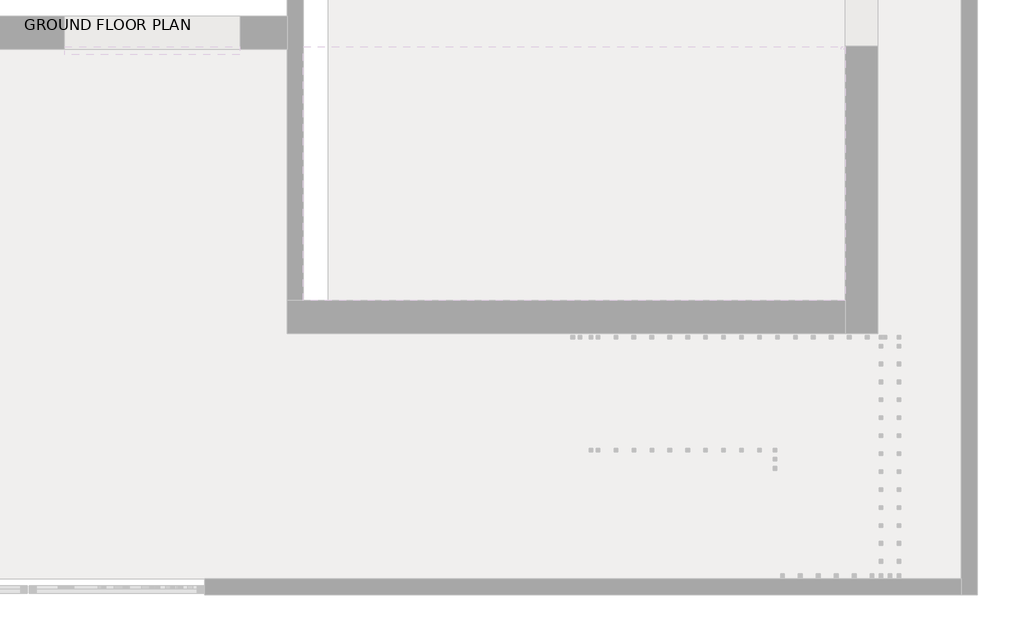
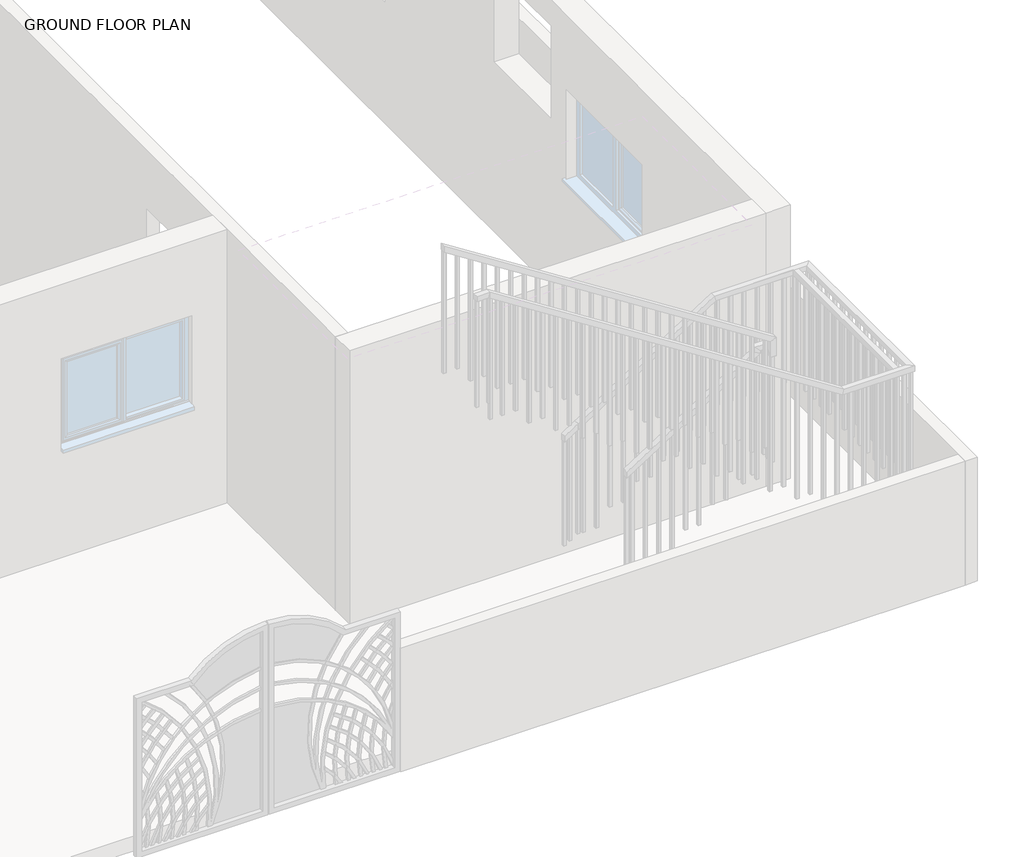
# One storey, part 16 of 23: 2 railings.
"""IFC4 building model written with IfcOpenShell, lengths in millimetres."""

from ifc_helpers import new_model, si_unit, frame, origin, place, context, project, spatial, polyline, outline, extrude, faceted_brep, element, save

model = new_model("IFC4")

# Units and contexts
model_context = context("Model", 3, world=origin())
ifc_project = project(units=[si_unit("LENGTHUNIT", "METRE", prefix="MILLI")], contexts=[model_context])

# Site, building, storey
site = spatial("IfcSite", under=ifc_project)
building = spatial("IfcBuilding", under=site)
storey = spatial("IfcBuildingStorey", under=building, Name="GROUND FLOOR PLAN", Elevation=487.68)

# Railings
placement = place(None, origin())
element("IfcRailing", 1, ObjectType="1100mm", at=placement, inside=storey, context=model_context, shape_type="SolidModel", body=[
    faceted_brep([(-8680.149573, -10220.0521308, 1912.8), (-8680.149573, -10220.0521308, 1853.4423995), (-8680.149573, -10270.0521308, 1853.4423995), (-8680.149573, -10270.0521308, 1912.8), (-7409.7306254, -10220.0521308, 2725.6), (-7395.1045513, -10220.0521308, 2675.6), (-7395.1045513, -10270.0521308, 2675.6), (-7409.7306254, -10270.0521308, 2725.6), (-6495.8132565, -10220.0521308, 2725.6), (-6495.8132565, -10220.0521308, 2675.6), (-6545.8132565, -10270.0521308, 2675.6), (-6545.8132565, -10270.0521308, 2725.6), (-6495.8132565, -11933.6860066, 2725.6), (-6495.8132565, -11933.6860066, 2675.6), (-6545.8132565, -11883.6860066, 2675.6), (-6545.8132565, -11883.6860066, 2725.6), (-7155.718398, -11933.6860066, 2725.6), (-7170.3479429, -11933.6860066, 2675.6), (-7170.3479429, -11883.6860066, 2675.6), (-7155.718398, -11883.6860066, 2725.6), (-10457.8773536, -11933.6860066, 4838.88), (-10457.8773536, -11883.6860066, 4838.88), (-10457.8773536, -11883.6860066, 4779.517542), (-10457.8773536, -11933.6860066, 4779.517542)], [[[0, 1, 2, 3]], [[1, 0, 4, 5]], [[2, 1, 5, 6]], [[3, 2, 6, 7]], [[0, 3, 7, 4]], [[5, 4, 8, 9]], [[6, 5, 9, 10]], [[7, 6, 10, 11]], [[4, 7, 11, 8]], [[9, 8, 12, 13]], [[10, 9, 13, 14]], [[11, 10, 14, 15]], [[8, 11, 15, 12]], [[13, 12, 16, 17]], [[14, 13, 17, 18]], [[15, 14, 18, 19]], [[12, 15, 19, 16]], [[20, 21, 22, 23]], [[17, 16, 20, 23]], [[18, 17, 23, 22]], [[19, 18, 22, 21]], [[16, 19, 21, 20]]]),
    extrude(outline(polyline([(4691.8007425, -10320.8132565), (4707.7999723, -10345.8132565), (3576.32, -10345.8132565), (3576.32, -10320.8132565), (4691.8007425, -10320.8132565)])), frame((0.0, -11921.1860066, 0.0), z_axis=(0.0, 1.0, 0.0), x_axis=(0.0, 0.0, 1.0)), (0.0, 0.0, 1.0), 25.0),
    extrude(outline(polyline([(4611.8045935, -10195.8132565), (4627.8038233, -10220.8132565), (3576.32, -10220.8132565), (3576.32, -10195.8132565), (4611.8045935, -10195.8132565)])), frame((0.0, -11921.1860066, 0.0), z_axis=(0.0, 1.0, 0.0), x_axis=(0.0, 0.0, 1.0)), (0.0, 0.0, 1.0), 25.0),
    extrude(outline(polyline([(4531.8084444, -10070.8132565), (4547.8076742, -10095.8132565), (3413.76, -10095.8132565), (3413.76, -10070.8132565), (4531.8084444, -10070.8132565)])), frame((0.0, -11921.1860066, 0.0), z_axis=(0.0, 1.0, 0.0), x_axis=(0.0, 0.0, 1.0)), (0.0, 0.0, 1.0), 25.0),
    extrude(outline(polyline([(4451.8122954, -9945.8132565), (4467.8115252, -9970.8132565), (3413.76, -9970.8132565), (3413.76, -9945.8132565), (4451.8122954, -9945.8132565)])), frame((0.0, -11921.1860066, 0.0), z_axis=(0.0, 1.0, 0.0), x_axis=(0.0, 0.0, 1.0)), (0.0, 0.0, 1.0), 25.0),
    extrude(outline(polyline([(4371.8161463, -9820.8132565), (4387.8153761, -9845.8132565), (3251.2, -9845.8132565), (3251.2, -9820.8132565), (4371.8161463, -9820.8132565)])), frame((0.0, -11921.1860066, 0.0), z_axis=(0.0, 1.0, 0.0), x_axis=(0.0, 0.0, 1.0)), (0.0, 0.0, 1.0), 25.0),
    extrude(outline(polyline([(4291.8423995, -9695.8132565), (4307.8371231, -9720.8132565), (3251.2, -9720.8132565), (3251.2, -9695.8132565), (4291.8423995, -9695.8132565)])), frame((0.0, -11921.1860066, 0.0), z_axis=(0.0, 1.0, 0.0), x_axis=(0.0, 0.0, 1.0)), (0.0, 0.0, 1.0), 25.0),
    extrude(outline(polyline([(4211.8238482, -9570.8132565), (4227.823078, -9595.8132565), (3088.64, -9595.8132565), (3088.64, -9570.8132565), (4211.8238482, -9570.8132565)])), frame((0.0, -11921.1860066, 0.0), z_axis=(0.0, 1.0, 0.0), x_axis=(0.0, 0.0, 1.0)), (0.0, 0.0, 1.0), 25.0),
    extrude(outline(polyline([(4131.8276992, -9445.8132565), (4147.826929, -9470.8132565), (3088.64, -9470.8132565), (3088.64, -9445.8132565), (4131.8276992, -9445.8132565)])), frame((0.0, -11921.1860066, 0.0), z_axis=(0.0, 1.0, 0.0), x_axis=(0.0, 0.0, 1.0)), (0.0, 0.0, 1.0), 25.0),
    extrude(outline(polyline([(4051.8315501, -9320.8132565), (4067.8307799, -9345.8132565), (2926.08, -9345.8132565), (2926.08, -9320.8132565), (4051.8315501, -9320.8132565)])), frame((0.0, -11921.1860066, 0.0), z_axis=(0.0, 1.0, 0.0), x_axis=(0.0, 0.0, 1.0)), (0.0, 0.0, 1.0), 25.0),
    extrude(outline(polyline([(3971.835401, -9195.8132565), (3987.8346309, -9220.8132565), (2926.08, -9220.8132565), (2926.08, -9195.8132565), (3971.835401, -9195.8132565)])), frame((0.0, -11921.1860066, 0.0), z_axis=(0.0, 1.0, 0.0), x_axis=(0.0, 0.0, 1.0)), (0.0, 0.0, 1.0), 25.0),
    extrude(outline(polyline([(3891.839252, -9070.8132565), (3907.8384818, -9095.8132565), (2763.52, -9095.8132565), (2763.52, -9070.8132565), (3891.839252, -9070.8132565)])), frame((0.0, -11921.1860066, 0.0), z_axis=(0.0, 1.0, 0.0), x_axis=(0.0, 0.0, 1.0)), (0.0, 0.0, 1.0), 25.0),
    extrude(outline(polyline([(3811.8431029, -8945.8132565), (3827.8423328, -8970.8132565), (2763.52, -8970.8132565), (2763.52, -8945.8132565), (3811.8431029, -8945.8132565)])), frame((0.0, -11921.1860066, 0.0), z_axis=(0.0, 1.0, 0.0), x_axis=(0.0, 0.0, 1.0)), (0.0, 0.0, 1.0), 25.0),
    extrude(outline(polyline([(3731.8469539, -8820.8132565), (3747.8461837, -8845.8132565), (2600.96, -8845.8132565), (2600.96, -8820.8132565), (3731.8469539, -8820.8132565)])), frame((0.0, -11921.1860066, 0.0), z_axis=(0.0, 1.0, 0.0), x_axis=(0.0, 0.0, 1.0)), (0.0, 0.0, 1.0), 25.0),
    extrude(outline(polyline([(3651.8508048, -8695.8132565), (3667.8500347, -8720.8132565), (2600.96, -8720.8132565), (2600.96, -8695.8132565), (3651.8508048, -8695.8132565)])), frame((0.0, -11921.1860066, 0.0), z_axis=(0.0, 1.0, 0.0), x_axis=(0.0, 0.0, 1.0)), (0.0, 0.0, 1.0), 25.0),
    extrude(outline(polyline([(3571.8546558, -8570.8132565), (3587.8538856, -8595.8132565), (2438.4, -8595.8132565), (2438.4, -8570.8132565), (3571.8546558, -8570.8132565)])), frame((0.0, -11921.1860066, 0.0), z_axis=(0.0, 1.0, 0.0), x_axis=(0.0, 0.0, 1.0)), (0.0, 0.0, 1.0), 25.0),
    extrude(outline(polyline([(3491.8585067, -8445.8132565), (3507.8577365, -8470.8132565), (2438.4, -8470.8132565), (2438.4, -8445.8132565), (3491.8585067, -8445.8132565)])), frame((0.0, -11921.1860066, 0.0), z_axis=(0.0, 1.0, 0.0), x_axis=(0.0, 0.0, 1.0)), (0.0, 0.0, 1.0), 25.0),
    extrude(outline(polyline([(3411.8623577, -8320.8132565), (3427.8615875, -8345.8132565), (2275.84, -8345.8132565), (2275.84, -8320.8132565), (3411.8623577, -8320.8132565)])), frame((0.0, -11921.1860066, 0.0), z_axis=(0.0, 1.0, 0.0), x_axis=(0.0, 0.0, 1.0)), (0.0, 0.0, 1.0), 25.0),
    extrude(outline(polyline([(3331.8662086, -8195.8132565), (3347.8654384, -8220.8132565), (2275.84, -8220.8132565), (2275.84, -8195.8132565), (3331.8662086, -8195.8132565)])), frame((0.0, -11921.1860066, 0.0), z_axis=(0.0, 1.0, 0.0), x_axis=(0.0, 0.0, 1.0)), (0.0, 0.0, 1.0), 25.0),
    extrude(outline(polyline([(3251.8700596, -8070.8132565), (3267.8692894, -8095.8132565), (2113.28, -8095.8132565), (2113.28, -8070.8132565), (3251.8700596, -8070.8132565)])), frame((0.0, -11921.1860066, 0.0), z_axis=(0.0, 1.0, 0.0), x_axis=(0.0, 0.0, 1.0)), (0.0, 0.0, 1.0), 25.0),
    extrude(outline(polyline([(3171.8739105, -7945.8132565), (3187.8731403, -7970.8132565), (2113.28, -7970.8132565), (2113.28, -7945.8132565), (3171.8739105, -7945.8132565)])), frame((0.0, -11921.1860066, 0.0), z_axis=(0.0, 1.0, 0.0), x_axis=(0.0, 0.0, 1.0)), (0.0, 0.0, 1.0), 25.0),
    extrude(outline(polyline([(3091.8777615, -7820.8132565), (3107.8769913, -7845.8132565), (1950.72, -7845.8132565), (1950.72, -7820.8132565), (3091.8777615, -7820.8132565)])), frame((0.0, -11921.1860066, 0.0), z_axis=(0.0, 1.0, 0.0), x_axis=(0.0, 0.0, 1.0)), (0.0, 0.0, 1.0), 25.0),
    extrude(outline(polyline([(3011.8816124, -7695.8132565), (3027.8808422, -7720.8132565), (1950.72, -7720.8132565), (1950.72, -7695.8132565), (3011.8816124, -7695.8132565)])), frame((0.0, -11921.1860066, 0.0), z_axis=(0.0, 1.0, 0.0), x_axis=(0.0, 0.0, 1.0)), (0.0, 0.0, 1.0), 25.0),
    extrude(outline(polyline([(2931.8854634, -7570.8132565), (2947.8846932, -7595.8132565), (1788.16, -7595.8132565), (1788.16, -7570.8132565), (2931.8854634, -7570.8132565)])), frame((0.0, -11921.1860066, 0.0), z_axis=(0.0, 1.0, 0.0), x_axis=(0.0, 0.0, 1.0)), (0.0, 0.0, 1.0), 25.0),
    extrude(outline(polyline([(2851.8893143, -7445.8132565), (2867.8885441, -7470.8132565), (1788.16, -7470.8132565), (1788.16, -7445.8132565), (2851.8893143, -7445.8132565)])), frame((0.0, -11921.1860066, 0.0), z_axis=(0.0, 1.0, 0.0), x_axis=(0.0, 0.0, 1.0)), (0.0, 0.0, 1.0), 25.0),
    extrude(outline(polyline([(2771.8931653, -7320.8132565), (2787.8923951, -7345.8132565), (1625.6, -7345.8132565), (1625.6, -7320.8132565), (2771.8931653, -7320.8132565)])), frame((0.0, -11921.1860066, 0.0), z_axis=(0.0, 1.0, 0.0), x_axis=(0.0, 0.0, 1.0)), (0.0, 0.0, 1.0), 25.0),
    extrude(outline(polyline([(2691.8970162, -7195.8132565), (2707.896246, -7220.8132565), (1625.6, -7220.8132565), (1625.6, -7195.8132565), (2691.8970162, -7195.8132565)])), frame((0.0, -11921.1860066, 0.0), z_axis=(0.0, 1.0, 0.0), x_axis=(0.0, 0.0, 1.0)), (0.0, 0.0, 1.0), 25.0),
    extrude(outline(polyline([(-7070.8132565, -11921.1860066), (-7095.8132565, -11921.1860066), (-7095.8132565, -11896.1860066), (-7070.8132565, -11896.1860066), (-7070.8132565, -11921.1860066)])), frame((0.0, 0.0, 1625.6), z_axis=(0.0, 0.0, 1.0), x_axis=(1.0, 0.0, 0.0)), (0.0, 0.0, 1.0), 1050.0),
    extrude(outline(polyline([(-6945.8132565, -11921.1860066), (-6970.8132565, -11921.1860066), (-6970.8132565, -11896.1860066), (-6945.8132565, -11896.1860066), (-6945.8132565, -11921.1860066)])), frame((0.0, 0.0, 1625.6), z_axis=(0.0, 0.0, 1.0), x_axis=(1.0, 0.0, 0.0)), (0.0, 0.0, 1.0), 1050.0),
    extrude(outline(polyline([(-6820.8132565, -11921.1860066), (-6845.8132565, -11921.1860066), (-6845.8132565, -11896.1860066), (-6820.8132565, -11896.1860066), (-6820.8132565, -11921.1860066)])), frame((0.0, 0.0, 1625.6), z_axis=(0.0, 0.0, 1.0), x_axis=(1.0, 0.0, 0.0)), (0.0, 0.0, 1.0), 1050.0),
    extrude(outline(polyline([(-6695.8132565, -11921.1860066), (-6720.8132565, -11921.1860066), (-6720.8132565, -11896.1860066), (-6695.8132565, -11896.1860066), (-6695.8132565, -11921.1860066)])), frame((0.0, 0.0, 1625.6), z_axis=(0.0, 0.0, 1.0), x_axis=(1.0, 0.0, 0.0)), (0.0, 0.0, 1.0), 1050.0),
    extrude(outline(polyline([(-6570.8132565, -11921.1860066), (-6595.8132565, -11921.1860066), (-6595.8132565, -11896.1860066), (-6570.8132565, -11896.1860066), (-6570.8132565, -11921.1860066)])), frame((0.0, 0.0, 1625.6), z_axis=(0.0, 0.0, 1.0), x_axis=(1.0, 0.0, 0.0)), (0.0, 0.0, 1.0), 1050.0),
    extrude(outline(polyline([(-6508.3132565, -11795.0521308), (-6508.3132565, -11820.0521308), (-6533.3132565, -11820.0521308), (-6533.3132565, -11795.0521308), (-6508.3132565, -11795.0521308)])), frame((0.0, 0.0, 1625.6), z_axis=(0.0, 0.0, 1.0), x_axis=(1.0, 0.0, 0.0)), (0.0, 0.0, 1.0), 1050.0),
    extrude(outline(polyline([(-6508.3132565, -11670.0521308), (-6508.3132565, -11695.0521308), (-6533.3132565, -11695.0521308), (-6533.3132565, -11670.0521308), (-6508.3132565, -11670.0521308)])), frame((0.0, 0.0, 1625.6), z_axis=(0.0, 0.0, 1.0), x_axis=(1.0, 0.0, 0.0)), (0.0, 0.0, 1.0), 1050.0),
    extrude(outline(polyline([(-6508.3132565, -11545.0521308), (-6508.3132565, -11570.0521308), (-6533.3132565, -11570.0521308), (-6533.3132565, -11545.0521308), (-6508.3132565, -11545.0521308)])), frame((0.0, 0.0, 1625.6), z_axis=(0.0, 0.0, 1.0), x_axis=(1.0, 0.0, 0.0)), (0.0, 0.0, 1.0), 1050.0),
    extrude(outline(polyline([(-6508.3132565, -11420.0521308), (-6508.3132565, -11445.0521308), (-6533.3132565, -11445.0521308), (-6533.3132565, -11420.0521308), (-6508.3132565, -11420.0521308)])), frame((0.0, 0.0, 1625.6), z_axis=(0.0, 0.0, 1.0), x_axis=(1.0, 0.0, 0.0)), (0.0, 0.0, 1.0), 1050.0),
    extrude(outline(polyline([(-6508.3132565, -11295.0521308), (-6508.3132565, -11320.0521308), (-6533.3132565, -11320.0521308), (-6533.3132565, -11295.0521308), (-6508.3132565, -11295.0521308)])), frame((0.0, 0.0, 1625.6), z_axis=(0.0, 0.0, 1.0), x_axis=(1.0, 0.0, 0.0)), (0.0, 0.0, 1.0), 1050.0),
    extrude(outline(polyline([(-6508.3132565, -11170.0521308), (-6508.3132565, -11195.0521308), (-6533.3132565, -11195.0521308), (-6533.3132565, -11170.0521308), (-6508.3132565, -11170.0521308)])), frame((0.0, 0.0, 1625.6), z_axis=(0.0, 0.0, 1.0), x_axis=(1.0, 0.0, 0.0)), (0.0, 0.0, 1.0), 1050.0),
    extrude(outline(polyline([(-6508.3132565, -11045.0521308), (-6508.3132565, -11070.0521308), (-6533.3132565, -11070.0521308), (-6533.3132565, -11045.0521308), (-6508.3132565, -11045.0521308)])), frame((0.0, 0.0, 1625.6), z_axis=(0.0, 0.0, 1.0), x_axis=(1.0, 0.0, 0.0)), (0.0, 0.0, 1.0), 1050.0),
    extrude(outline(polyline([(-6508.3132565, -10920.0521308), (-6508.3132565, -10945.0521308), (-6533.3132565, -10945.0521308), (-6533.3132565, -10920.0521308), (-6508.3132565, -10920.0521308)])), frame((0.0, 0.0, 1625.6), z_axis=(0.0, 0.0, 1.0), x_axis=(1.0, 0.0, 0.0)), (0.0, 0.0, 1.0), 1050.0),
    extrude(outline(polyline([(-6508.3132565, -10795.0521308), (-6508.3132565, -10820.0521308), (-6533.3132565, -10820.0521308), (-6533.3132565, -10795.0521308), (-6508.3132565, -10795.0521308)])), frame((0.0, 0.0, 1625.6), z_axis=(0.0, 0.0, 1.0), x_axis=(1.0, 0.0, 0.0)), (0.0, 0.0, 1.0), 1050.0),
    extrude(outline(polyline([(-6508.3132565, -10670.0521308), (-6508.3132565, -10695.0521308), (-6533.3132565, -10695.0521308), (-6533.3132565, -10670.0521308), (-6508.3132565, -10670.0521308)])), frame((0.0, 0.0, 1625.6), z_axis=(0.0, 0.0, 1.0), x_axis=(1.0, 0.0, 0.0)), (0.0, 0.0, 1.0), 1050.0),
    extrude(outline(polyline([(-6508.3132565, -10545.0521308), (-6508.3132565, -10570.0521308), (-6533.3132565, -10570.0521308), (-6533.3132565, -10545.0521308), (-6508.3132565, -10545.0521308)])), frame((0.0, 0.0, 1625.6), z_axis=(0.0, 0.0, 1.0), x_axis=(1.0, 0.0, 0.0)), (0.0, 0.0, 1.0), 1050.0),
    extrude(outline(polyline([(-6508.3132565, -10420.0521308), (-6508.3132565, -10445.0521308), (-6533.3132565, -10445.0521308), (-6533.3132565, -10420.0521308), (-6508.3132565, -10420.0521308)])), frame((0.0, 0.0, 1625.6), z_axis=(0.0, 0.0, 1.0), x_axis=(1.0, 0.0, 0.0)), (0.0, 0.0, 1.0), 1050.0),
    extrude(outline(polyline([(-6508.3132565, -10295.0521308), (-6508.3132565, -10320.0521308), (-6533.3132565, -10320.0521308), (-6533.3132565, -10295.0521308), (-6508.3132565, -10295.0521308)])), frame((0.0, 0.0, 1625.6), z_axis=(0.0, 0.0, 1.0), x_axis=(1.0, 0.0, 0.0)), (0.0, 0.0, 1.0), 1050.0),
    extrude(outline(polyline([(-6630.149573, -10232.5521308), (-6605.149573, -10232.5521308), (-6605.149573, -10257.5521308), (-6630.149573, -10257.5521308), (-6630.149573, -10232.5521308)])), frame((0.0, 0.0, 1625.6), z_axis=(0.0, 0.0, 1.0), x_axis=(1.0, 0.0, 0.0)), (0.0, 0.0, 1.0), 1050.0),
    extrude(outline(polyline([(-6755.149573, -10232.5521308), (-6730.149573, -10232.5521308), (-6730.149573, -10257.5521308), (-6755.149573, -10257.5521308), (-6755.149573, -10232.5521308)])), frame((0.0, 0.0, 1625.6), z_axis=(0.0, 0.0, 1.0), x_axis=(1.0, 0.0, 0.0)), (0.0, 0.0, 1.0), 1050.0),
    extrude(outline(polyline([(-6880.149573, -10232.5521308), (-6855.149573, -10232.5521308), (-6855.149573, -10257.5521308), (-6880.149573, -10257.5521308), (-6880.149573, -10232.5521308)])), frame((0.0, 0.0, 1625.6), z_axis=(0.0, 0.0, 1.0), x_axis=(1.0, 0.0, 0.0)), (0.0, 0.0, 1.0), 1050.0),
    extrude(outline(polyline([(-7005.149573, -10232.5521308), (-6980.149573, -10232.5521308), (-6980.149573, -10257.5521308), (-7005.149573, -10257.5521308), (-7005.149573, -10232.5521308)])), frame((0.0, 0.0, 1625.6), z_axis=(0.0, 0.0, 1.0), x_axis=(1.0, 0.0, 0.0)), (0.0, 0.0, 1.0), 1050.0),
    extrude(outline(polyline([(-7130.149573, -10232.5521308), (-7105.149573, -10232.5521308), (-7105.149573, -10257.5521308), (-7130.149573, -10257.5521308), (-7130.149573, -10232.5521308)])), frame((0.0, 0.0, 1625.6), z_axis=(0.0, 0.0, 1.0), x_axis=(1.0, 0.0, 0.0)), (0.0, 0.0, 1.0), 1050.0),
    extrude(outline(polyline([(-7255.149573, -10232.5521308), (-7230.149573, -10232.5521308), (-7230.149573, -10257.5521308), (-7255.149573, -10257.5521308), (-7255.149573, -10232.5521308)])), frame((0.0, 0.0, 1625.6), z_axis=(0.0, 0.0, 1.0), x_axis=(1.0, 0.0, 0.0)), (0.0, 0.0, 1.0), 1050.0),
    extrude(outline(polyline([(-7380.149573, -10232.5521308), (-7355.149573, -10232.5521308), (-7355.149573, -10257.5521308), (-7380.149573, -10257.5521308), (-7380.149573, -10232.5521308)])), frame((0.0, 0.0, 1625.6), z_axis=(0.0, 0.0, 1.0), x_axis=(1.0, 0.0, 0.0)), (0.0, 0.0, 1.0), 1050.0),
    extrude(outline(polyline([(1463.04, -7505.149573), (1463.04, -7480.149573), (2621.1891352, -7480.149573), (2605.1944115, -7505.149573), (1463.04, -7505.149573)])), frame((0.0, -10257.5521308, 0.0), z_axis=(0.0, 1.0, 0.0), x_axis=(0.0, 0.0, 1.0)), (0.0, 0.0, 1.0), 25.0),
    extrude(outline(polyline([(1463.04, -7630.149573), (1463.04, -7605.149573), (2541.2155169, -7605.149573), (2525.2207932, -7630.149573), (1463.04, -7630.149573)])), frame((0.0, -10257.5521308, 0.0), z_axis=(0.0, 1.0, 0.0), x_axis=(0.0, 0.0, 1.0)), (0.0, 0.0, 1.0), 25.0),
    extrude(outline(polyline([(1300.48, -7755.149573), (1300.48, -7730.149573), (2461.2418986, -7730.149573), (2445.2471749, -7755.149573), (1300.48, -7755.149573)])), frame((0.0, -10257.5521308, 0.0), z_axis=(0.0, 1.0, 0.0), x_axis=(0.0, 0.0, 1.0)), (0.0, 0.0, 1.0), 25.0),
    extrude(outline(polyline([(1300.48, -7880.149573), (1300.48, -7855.149573), (2381.2682803, -7855.149573), (2365.2735566, -7880.149573), (1300.48, -7880.149573)])), frame((0.0, -10257.5521308, 0.0), z_axis=(0.0, 1.0, 0.0), x_axis=(0.0, 0.0, 1.0)), (0.0, 0.0, 1.0), 25.0),
    extrude(outline(polyline([(1137.92, -8005.149573), (1137.92, -7980.149573), (2301.294662, -7980.149573), (2285.2999383, -8005.149573), (1137.92, -8005.149573)])), frame((0.0, -10257.5521308, 0.0), z_axis=(0.0, 1.0, 0.0), x_axis=(0.0, 0.0, 1.0)), (0.0, 0.0, 1.0), 25.0),
    extrude(outline(polyline([(1137.92, -8130.149573), (1137.92, -8105.149573), (2221.3210437, -8105.149573), (2205.32632, -8130.149573), (1137.92, -8130.149573)])), frame((0.0, -10257.5521308, 0.0), z_axis=(0.0, 1.0, 0.0), x_axis=(0.0, 0.0, 1.0)), (0.0, 0.0, 1.0), 25.0),
    extrude(outline(polyline([(975.36, -8255.149573), (975.36, -8230.149573), (2141.3474254, -8230.149573), (2125.3527017, -8255.149573), (975.36, -8255.149573)])), frame((0.0, -10257.5521308, 0.0), z_axis=(0.0, 1.0, 0.0), x_axis=(0.0, 0.0, 1.0)), (0.0, 0.0, 1.0), 25.0),
    extrude(outline(polyline([(975.36, -8380.149573), (975.36, -8355.149573), (2061.3738071, -8355.149573), (2045.3790834, -8380.149573), (975.36, -8380.149573)])), frame((0.0, -10257.5521308, 0.0), z_axis=(0.0, 1.0, 0.0), x_axis=(0.0, 0.0, 1.0)), (0.0, 0.0, 1.0), 25.0),
    extrude(outline(polyline([(812.8, -8505.149573), (812.8, -8480.149573), (1981.4001888, -8480.149573), (1965.4054651, -8505.149573), (812.8, -8505.149573)])), frame((0.0, -10257.5521308, 0.0), z_axis=(0.0, 1.0, 0.0), x_axis=(0.0, 0.0, 1.0)), (0.0, 0.0, 1.0), 25.0),
    extrude(outline(polyline([(812.8, -8630.149573), (812.8, -8605.149573), (1901.4265705, -8605.149573), (1885.4318468, -8630.149573), (812.8, -8630.149573)])), frame((0.0, -10257.5521308, 0.0), z_axis=(0.0, 1.0, 0.0), x_axis=(0.0, 0.0, 1.0)), (0.0, 0.0, 1.0), 25.0),
    extrude(outline(polyline([(-6508.3132565, -11896.1860066), (-6508.3132565, -11921.1860066), (-6533.3132565, -11921.1860066), (-6533.3132565, -11896.1860066), (-6508.3132565, -11896.1860066)])), frame((0.0, 0.0, 1625.6), z_axis=(0.0, 0.0, 1.0), x_axis=(1.0, 0.0, 0.0)), (0.0, 0.0, 1.0), 1050.0),
    extrude(outline(polyline([(-6533.3132565, -10232.5521308), (-6508.3132565, -10232.5521308), (-6508.3132565, -10257.5521308), (-6533.3132565, -10257.5521308), (-6533.3132565, -10232.5521308)])), frame((0.0, 0.0, 1625.6), z_axis=(0.0, 0.0, 1.0), x_axis=(1.0, 0.0, 0.0)), (0.0, 0.0, 1.0), 1050.0),
    extrude(outline(polyline([(4763.5183122, -10432.8773536), (4779.517542, -10457.8773536), (3576.32, -10457.8773536), (3576.32, -10432.8773536), (4763.5183122, -10432.8773536)])), frame((0.0, -11921.1860066, 0.0), z_axis=(0.0, 1.0, 0.0), x_axis=(0.0, 0.0, 1.0)), (0.0, 0.0, 1.0), 25.0),
    extrude(outline(polyline([(812.8, -8680.149573), (812.8, -8655.149573), (1869.4371231, -8655.149573), (1853.4423995, -8680.149573), (812.8, -8680.149573)])), frame((0.0, -10257.5521308, 0.0), z_axis=(0.0, 1.0, 0.0), x_axis=(0.0, 0.0, 1.0)), (0.0, 0.0, 1.0), 25.0),
])
element("IfcRailing", 2, ObjectType="1100mm", at=placement, inside=storey, context=model_context, shape_type="SolidModel", body=[
    faceted_brep([(-8680.149573, -10220.0521308, 1912.8), (-8680.149573, -10220.0521308, 1853.4423995), (-8680.149573, -10270.0521308, 1853.4423995), (-8680.149573, -10270.0521308, 1912.8), (-7409.7306254, -10220.0521308, 2725.6), (-7395.1045513, -10220.0521308, 2675.6), (-7395.1045513, -10270.0521308, 2675.6), (-7409.7306254, -10270.0521308, 2725.6), (-6495.8132565, -10220.0521308, 2725.6), (-6495.8132565, -10220.0521308, 2675.6), (-6545.8132565, -10270.0521308, 2675.6), (-6545.8132565, -10270.0521308, 2725.6), (-6495.8132565, -11933.6860066, 2725.6), (-6495.8132565, -11933.6860066, 2675.6), (-6545.8132565, -11883.6860066, 2675.6), (-6545.8132565, -11883.6860066, 2725.6), (-7155.718398, -11933.6860066, 2725.6), (-7170.3479429, -11933.6860066, 2675.6), (-7170.3479429, -11883.6860066, 2675.6), (-7155.718398, -11883.6860066, 2725.6), (-10457.8773536, -11933.6860066, 4838.88), (-10457.8773536, -11883.6860066, 4838.88), (-10457.8773536, -11883.6860066, 4779.517542), (-10457.8773536, -11933.6860066, 4779.517542)], [[[0, 1, 2, 3]], [[1, 0, 4, 5]], [[2, 1, 5, 6]], [[3, 2, 6, 7]], [[0, 3, 7, 4]], [[5, 4, 8, 9]], [[6, 5, 9, 10]], [[7, 6, 10, 11]], [[4, 7, 11, 8]], [[9, 8, 12, 13]], [[10, 9, 13, 14]], [[11, 10, 14, 15]], [[8, 11, 15, 12]], [[13, 12, 16, 17]], [[14, 13, 17, 18]], [[15, 14, 18, 19]], [[12, 15, 19, 16]], [[20, 21, 22, 23]], [[17, 16, 20, 23]], [[18, 17, 23, 22]], [[19, 18, 22, 21]], [[16, 19, 21, 20]]]),
    extrude(outline(polyline([(4691.8007425, -10320.8132565), (4707.7999723, -10345.8132565), (3576.32, -10345.8132565), (3576.32, -10320.8132565), (4691.8007425, -10320.8132565)])), frame((0.0, -11921.1860066, 0.0), z_axis=(0.0, 1.0, 0.0), x_axis=(0.0, 0.0, 1.0)), (0.0, 0.0, 1.0), 25.0),
    extrude(outline(polyline([(4611.8045935, -10195.8132565), (4627.8038233, -10220.8132565), (3576.32, -10220.8132565), (3576.32, -10195.8132565), (4611.8045935, -10195.8132565)])), frame((0.0, -11921.1860066, 0.0), z_axis=(0.0, 1.0, 0.0), x_axis=(0.0, 0.0, 1.0)), (0.0, 0.0, 1.0), 25.0),
    extrude(outline(polyline([(4531.8084444, -10070.8132565), (4547.8076742, -10095.8132565), (3413.76, -10095.8132565), (3413.76, -10070.8132565), (4531.8084444, -10070.8132565)])), frame((0.0, -11921.1860066, 0.0), z_axis=(0.0, 1.0, 0.0), x_axis=(0.0, 0.0, 1.0)), (0.0, 0.0, 1.0), 25.0),
    extrude(outline(polyline([(4451.8122954, -9945.8132565), (4467.8115252, -9970.8132565), (3413.76, -9970.8132565), (3413.76, -9945.8132565), (4451.8122954, -9945.8132565)])), frame((0.0, -11921.1860066, 0.0), z_axis=(0.0, 1.0, 0.0), x_axis=(0.0, 0.0, 1.0)), (0.0, 0.0, 1.0), 25.0),
    extrude(outline(polyline([(4371.8161463, -9820.8132565), (4387.8153761, -9845.8132565), (3251.2, -9845.8132565), (3251.2, -9820.8132565), (4371.8161463, -9820.8132565)])), frame((0.0, -11921.1860066, 0.0), z_axis=(0.0, 1.0, 0.0), x_axis=(0.0, 0.0, 1.0)), (0.0, 0.0, 1.0), 25.0),
    extrude(outline(polyline([(4291.8423995, -9695.8132565), (4307.8371231, -9720.8132565), (3251.2, -9720.8132565), (3251.2, -9695.8132565), (4291.8423995, -9695.8132565)])), frame((0.0, -11921.1860066, 0.0), z_axis=(0.0, 1.0, 0.0), x_axis=(0.0, 0.0, 1.0)), (0.0, 0.0, 1.0), 25.0),
    extrude(outline(polyline([(4211.8238482, -9570.8132565), (4227.823078, -9595.8132565), (3088.64, -9595.8132565), (3088.64, -9570.8132565), (4211.8238482, -9570.8132565)])), frame((0.0, -11921.1860066, 0.0), z_axis=(0.0, 1.0, 0.0), x_axis=(0.0, 0.0, 1.0)), (0.0, 0.0, 1.0), 25.0),
    extrude(outline(polyline([(4131.8276992, -9445.8132565), (4147.826929, -9470.8132565), (3088.64, -9470.8132565), (3088.64, -9445.8132565), (4131.8276992, -9445.8132565)])), frame((0.0, -11921.1860066, 0.0), z_axis=(0.0, 1.0, 0.0), x_axis=(0.0, 0.0, 1.0)), (0.0, 0.0, 1.0), 25.0),
    extrude(outline(polyline([(4051.8315501, -9320.8132565), (4067.8307799, -9345.8132565), (2926.08, -9345.8132565), (2926.08, -9320.8132565), (4051.8315501, -9320.8132565)])), frame((0.0, -11921.1860066, 0.0), z_axis=(0.0, 1.0, 0.0), x_axis=(0.0, 0.0, 1.0)), (0.0, 0.0, 1.0), 25.0),
    extrude(outline(polyline([(3971.835401, -9195.8132565), (3987.8346309, -9220.8132565), (2926.08, -9220.8132565), (2926.08, -9195.8132565), (3971.835401, -9195.8132565)])), frame((0.0, -11921.1860066, 0.0), z_axis=(0.0, 1.0, 0.0), x_axis=(0.0, 0.0, 1.0)), (0.0, 0.0, 1.0), 25.0),
    extrude(outline(polyline([(3891.839252, -9070.8132565), (3907.8384818, -9095.8132565), (2763.52, -9095.8132565), (2763.52, -9070.8132565), (3891.839252, -9070.8132565)])), frame((0.0, -11921.1860066, 0.0), z_axis=(0.0, 1.0, 0.0), x_axis=(0.0, 0.0, 1.0)), (0.0, 0.0, 1.0), 25.0),
    extrude(outline(polyline([(3811.8431029, -8945.8132565), (3827.8423328, -8970.8132565), (2763.52, -8970.8132565), (2763.52, -8945.8132565), (3811.8431029, -8945.8132565)])), frame((0.0, -11921.1860066, 0.0), z_axis=(0.0, 1.0, 0.0), x_axis=(0.0, 0.0, 1.0)), (0.0, 0.0, 1.0), 25.0),
    extrude(outline(polyline([(3731.8469539, -8820.8132565), (3747.8461837, -8845.8132565), (2600.96, -8845.8132565), (2600.96, -8820.8132565), (3731.8469539, -8820.8132565)])), frame((0.0, -11921.1860066, 0.0), z_axis=(0.0, 1.0, 0.0), x_axis=(0.0, 0.0, 1.0)), (0.0, 0.0, 1.0), 25.0),
    extrude(outline(polyline([(3651.8508048, -8695.8132565), (3667.8500347, -8720.8132565), (2600.96, -8720.8132565), (2600.96, -8695.8132565), (3651.8508048, -8695.8132565)])), frame((0.0, -11921.1860066, 0.0), z_axis=(0.0, 1.0, 0.0), x_axis=(0.0, 0.0, 1.0)), (0.0, 0.0, 1.0), 25.0),
    extrude(outline(polyline([(3571.8546558, -8570.8132565), (3587.8538856, -8595.8132565), (2438.4, -8595.8132565), (2438.4, -8570.8132565), (3571.8546558, -8570.8132565)])), frame((0.0, -11921.1860066, 0.0), z_axis=(0.0, 1.0, 0.0), x_axis=(0.0, 0.0, 1.0)), (0.0, 0.0, 1.0), 25.0),
    extrude(outline(polyline([(3491.8585067, -8445.8132565), (3507.8577365, -8470.8132565), (2438.4, -8470.8132565), (2438.4, -8445.8132565), (3491.8585067, -8445.8132565)])), frame((0.0, -11921.1860066, 0.0), z_axis=(0.0, 1.0, 0.0), x_axis=(0.0, 0.0, 1.0)), (0.0, 0.0, 1.0), 25.0),
    extrude(outline(polyline([(3411.8623577, -8320.8132565), (3427.8615875, -8345.8132565), (2275.84, -8345.8132565), (2275.84, -8320.8132565), (3411.8623577, -8320.8132565)])), frame((0.0, -11921.1860066, 0.0), z_axis=(0.0, 1.0, 0.0), x_axis=(0.0, 0.0, 1.0)), (0.0, 0.0, 1.0), 25.0),
    extrude(outline(polyline([(3331.8662086, -8195.8132565), (3347.8654384, -8220.8132565), (2275.84, -8220.8132565), (2275.84, -8195.8132565), (3331.8662086, -8195.8132565)])), frame((0.0, -11921.1860066, 0.0), z_axis=(0.0, 1.0, 0.0), x_axis=(0.0, 0.0, 1.0)), (0.0, 0.0, 1.0), 25.0),
    extrude(outline(polyline([(3251.8700596, -8070.8132565), (3267.8692894, -8095.8132565), (2113.28, -8095.8132565), (2113.28, -8070.8132565), (3251.8700596, -8070.8132565)])), frame((0.0, -11921.1860066, 0.0), z_axis=(0.0, 1.0, 0.0), x_axis=(0.0, 0.0, 1.0)), (0.0, 0.0, 1.0), 25.0),
    extrude(outline(polyline([(3171.8739105, -7945.8132565), (3187.8731403, -7970.8132565), (2113.28, -7970.8132565), (2113.28, -7945.8132565), (3171.8739105, -7945.8132565)])), frame((0.0, -11921.1860066, 0.0), z_axis=(0.0, 1.0, 0.0), x_axis=(0.0, 0.0, 1.0)), (0.0, 0.0, 1.0), 25.0),
    extrude(outline(polyline([(3091.8777615, -7820.8132565), (3107.8769913, -7845.8132565), (1950.72, -7845.8132565), (1950.72, -7820.8132565), (3091.8777615, -7820.8132565)])), frame((0.0, -11921.1860066, 0.0), z_axis=(0.0, 1.0, 0.0), x_axis=(0.0, 0.0, 1.0)), (0.0, 0.0, 1.0), 25.0),
    extrude(outline(polyline([(3011.8816124, -7695.8132565), (3027.8808422, -7720.8132565), (1950.72, -7720.8132565), (1950.72, -7695.8132565), (3011.8816124, -7695.8132565)])), frame((0.0, -11921.1860066, 0.0), z_axis=(0.0, 1.0, 0.0), x_axis=(0.0, 0.0, 1.0)), (0.0, 0.0, 1.0), 25.0),
    extrude(outline(polyline([(2931.8854634, -7570.8132565), (2947.8846932, -7595.8132565), (1788.16, -7595.8132565), (1788.16, -7570.8132565), (2931.8854634, -7570.8132565)])), frame((0.0, -11921.1860066, 0.0), z_axis=(0.0, 1.0, 0.0), x_axis=(0.0, 0.0, 1.0)), (0.0, 0.0, 1.0), 25.0),
    extrude(outline(polyline([(2851.8893143, -7445.8132565), (2867.8885441, -7470.8132565), (1788.16, -7470.8132565), (1788.16, -7445.8132565), (2851.8893143, -7445.8132565)])), frame((0.0, -11921.1860066, 0.0), z_axis=(0.0, 1.0, 0.0), x_axis=(0.0, 0.0, 1.0)), (0.0, 0.0, 1.0), 25.0),
    extrude(outline(polyline([(2771.8931653, -7320.8132565), (2787.8923951, -7345.8132565), (1625.6, -7345.8132565), (1625.6, -7320.8132565), (2771.8931653, -7320.8132565)])), frame((0.0, -11921.1860066, 0.0), z_axis=(0.0, 1.0, 0.0), x_axis=(0.0, 0.0, 1.0)), (0.0, 0.0, 1.0), 25.0),
    extrude(outline(polyline([(2691.8970162, -7195.8132565), (2707.896246, -7220.8132565), (1625.6, -7220.8132565), (1625.6, -7195.8132565), (2691.8970162, -7195.8132565)])), frame((0.0, -11921.1860066, 0.0), z_axis=(0.0, 1.0, 0.0), x_axis=(0.0, 0.0, 1.0)), (0.0, 0.0, 1.0), 25.0),
    extrude(outline(polyline([(-7070.8132565, -11921.1860066), (-7095.8132565, -11921.1860066), (-7095.8132565, -11896.1860066), (-7070.8132565, -11896.1860066), (-7070.8132565, -11921.1860066)])), frame((0.0, 0.0, 1625.6), z_axis=(0.0, 0.0, 1.0), x_axis=(1.0, 0.0, 0.0)), (0.0, 0.0, 1.0), 1050.0),
    extrude(outline(polyline([(-6945.8132565, -11921.1860066), (-6970.8132565, -11921.1860066), (-6970.8132565, -11896.1860066), (-6945.8132565, -11896.1860066), (-6945.8132565, -11921.1860066)])), frame((0.0, 0.0, 1625.6), z_axis=(0.0, 0.0, 1.0), x_axis=(1.0, 0.0, 0.0)), (0.0, 0.0, 1.0), 1050.0),
    extrude(outline(polyline([(-6820.8132565, -11921.1860066), (-6845.8132565, -11921.1860066), (-6845.8132565, -11896.1860066), (-6820.8132565, -11896.1860066), (-6820.8132565, -11921.1860066)])), frame((0.0, 0.0, 1625.6), z_axis=(0.0, 0.0, 1.0), x_axis=(1.0, 0.0, 0.0)), (0.0, 0.0, 1.0), 1050.0),
    extrude(outline(polyline([(-6695.8132565, -11921.1860066), (-6720.8132565, -11921.1860066), (-6720.8132565, -11896.1860066), (-6695.8132565, -11896.1860066), (-6695.8132565, -11921.1860066)])), frame((0.0, 0.0, 1625.6), z_axis=(0.0, 0.0, 1.0), x_axis=(1.0, 0.0, 0.0)), (0.0, 0.0, 1.0), 1050.0),
    extrude(outline(polyline([(-6570.8132565, -11921.1860066), (-6595.8132565, -11921.1860066), (-6595.8132565, -11896.1860066), (-6570.8132565, -11896.1860066), (-6570.8132565, -11921.1860066)])), frame((0.0, 0.0, 1625.6), z_axis=(0.0, 0.0, 1.0), x_axis=(1.0, 0.0, 0.0)), (0.0, 0.0, 1.0), 1050.0),
    extrude(outline(polyline([(-6508.3132565, -11795.0521308), (-6508.3132565, -11820.0521308), (-6533.3132565, -11820.0521308), (-6533.3132565, -11795.0521308), (-6508.3132565, -11795.0521308)])), frame((0.0, 0.0, 1625.6), z_axis=(0.0, 0.0, 1.0), x_axis=(1.0, 0.0, 0.0)), (0.0, 0.0, 1.0), 1050.0),
    extrude(outline(polyline([(-6508.3132565, -11670.0521308), (-6508.3132565, -11695.0521308), (-6533.3132565, -11695.0521308), (-6533.3132565, -11670.0521308), (-6508.3132565, -11670.0521308)])), frame((0.0, 0.0, 1625.6), z_axis=(0.0, 0.0, 1.0), x_axis=(1.0, 0.0, 0.0)), (0.0, 0.0, 1.0), 1050.0),
    extrude(outline(polyline([(-6508.3132565, -11545.0521308), (-6508.3132565, -11570.0521308), (-6533.3132565, -11570.0521308), (-6533.3132565, -11545.0521308), (-6508.3132565, -11545.0521308)])), frame((0.0, 0.0, 1625.6), z_axis=(0.0, 0.0, 1.0), x_axis=(1.0, 0.0, 0.0)), (0.0, 0.0, 1.0), 1050.0),
    extrude(outline(polyline([(-6508.3132565, -11420.0521308), (-6508.3132565, -11445.0521308), (-6533.3132565, -11445.0521308), (-6533.3132565, -11420.0521308), (-6508.3132565, -11420.0521308)])), frame((0.0, 0.0, 1625.6), z_axis=(0.0, 0.0, 1.0), x_axis=(1.0, 0.0, 0.0)), (0.0, 0.0, 1.0), 1050.0),
    extrude(outline(polyline([(-6508.3132565, -11295.0521308), (-6508.3132565, -11320.0521308), (-6533.3132565, -11320.0521308), (-6533.3132565, -11295.0521308), (-6508.3132565, -11295.0521308)])), frame((0.0, 0.0, 1625.6), z_axis=(0.0, 0.0, 1.0), x_axis=(1.0, 0.0, 0.0)), (0.0, 0.0, 1.0), 1050.0),
    extrude(outline(polyline([(-6508.3132565, -11170.0521308), (-6508.3132565, -11195.0521308), (-6533.3132565, -11195.0521308), (-6533.3132565, -11170.0521308), (-6508.3132565, -11170.0521308)])), frame((0.0, 0.0, 1625.6), z_axis=(0.0, 0.0, 1.0), x_axis=(1.0, 0.0, 0.0)), (0.0, 0.0, 1.0), 1050.0),
    extrude(outline(polyline([(-6508.3132565, -11045.0521308), (-6508.3132565, -11070.0521308), (-6533.3132565, -11070.0521308), (-6533.3132565, -11045.0521308), (-6508.3132565, -11045.0521308)])), frame((0.0, 0.0, 1625.6), z_axis=(0.0, 0.0, 1.0), x_axis=(1.0, 0.0, 0.0)), (0.0, 0.0, 1.0), 1050.0),
    extrude(outline(polyline([(-6508.3132565, -10920.0521308), (-6508.3132565, -10945.0521308), (-6533.3132565, -10945.0521308), (-6533.3132565, -10920.0521308), (-6508.3132565, -10920.0521308)])), frame((0.0, 0.0, 1625.6), z_axis=(0.0, 0.0, 1.0), x_axis=(1.0, 0.0, 0.0)), (0.0, 0.0, 1.0), 1050.0),
    extrude(outline(polyline([(-6508.3132565, -10795.0521308), (-6508.3132565, -10820.0521308), (-6533.3132565, -10820.0521308), (-6533.3132565, -10795.0521308), (-6508.3132565, -10795.0521308)])), frame((0.0, 0.0, 1625.6), z_axis=(0.0, 0.0, 1.0), x_axis=(1.0, 0.0, 0.0)), (0.0, 0.0, 1.0), 1050.0),
    extrude(outline(polyline([(-6508.3132565, -10670.0521308), (-6508.3132565, -10695.0521308), (-6533.3132565, -10695.0521308), (-6533.3132565, -10670.0521308), (-6508.3132565, -10670.0521308)])), frame((0.0, 0.0, 1625.6), z_axis=(0.0, 0.0, 1.0), x_axis=(1.0, 0.0, 0.0)), (0.0, 0.0, 1.0), 1050.0),
    extrude(outline(polyline([(-6508.3132565, -10545.0521308), (-6508.3132565, -10570.0521308), (-6533.3132565, -10570.0521308), (-6533.3132565, -10545.0521308), (-6508.3132565, -10545.0521308)])), frame((0.0, 0.0, 1625.6), z_axis=(0.0, 0.0, 1.0), x_axis=(1.0, 0.0, 0.0)), (0.0, 0.0, 1.0), 1050.0),
    extrude(outline(polyline([(-6508.3132565, -10420.0521308), (-6508.3132565, -10445.0521308), (-6533.3132565, -10445.0521308), (-6533.3132565, -10420.0521308), (-6508.3132565, -10420.0521308)])), frame((0.0, 0.0, 1625.6), z_axis=(0.0, 0.0, 1.0), x_axis=(1.0, 0.0, 0.0)), (0.0, 0.0, 1.0), 1050.0),
    extrude(outline(polyline([(-6508.3132565, -10295.0521308), (-6508.3132565, -10320.0521308), (-6533.3132565, -10320.0521308), (-6533.3132565, -10295.0521308), (-6508.3132565, -10295.0521308)])), frame((0.0, 0.0, 1625.6), z_axis=(0.0, 0.0, 1.0), x_axis=(1.0, 0.0, 0.0)), (0.0, 0.0, 1.0), 1050.0),
    extrude(outline(polyline([(-6630.149573, -10232.5521308), (-6605.149573, -10232.5521308), (-6605.149573, -10257.5521308), (-6630.149573, -10257.5521308), (-6630.149573, -10232.5521308)])), frame((0.0, 0.0, 1625.6), z_axis=(0.0, 0.0, 1.0), x_axis=(1.0, 0.0, 0.0)), (0.0, 0.0, 1.0), 1050.0),
    extrude(outline(polyline([(-6755.149573, -10232.5521308), (-6730.149573, -10232.5521308), (-6730.149573, -10257.5521308), (-6755.149573, -10257.5521308), (-6755.149573, -10232.5521308)])), frame((0.0, 0.0, 1625.6), z_axis=(0.0, 0.0, 1.0), x_axis=(1.0, 0.0, 0.0)), (0.0, 0.0, 1.0), 1050.0),
    extrude(outline(polyline([(-6880.149573, -10232.5521308), (-6855.149573, -10232.5521308), (-6855.149573, -10257.5521308), (-6880.149573, -10257.5521308), (-6880.149573, -10232.5521308)])), frame((0.0, 0.0, 1625.6), z_axis=(0.0, 0.0, 1.0), x_axis=(1.0, 0.0, 0.0)), (0.0, 0.0, 1.0), 1050.0),
    extrude(outline(polyline([(-7005.149573, -10232.5521308), (-6980.149573, -10232.5521308), (-6980.149573, -10257.5521308), (-7005.149573, -10257.5521308), (-7005.149573, -10232.5521308)])), frame((0.0, 0.0, 1625.6), z_axis=(0.0, 0.0, 1.0), x_axis=(1.0, 0.0, 0.0)), (0.0, 0.0, 1.0), 1050.0),
    extrude(outline(polyline([(-7130.149573, -10232.5521308), (-7105.149573, -10232.5521308), (-7105.149573, -10257.5521308), (-7130.149573, -10257.5521308), (-7130.149573, -10232.5521308)])), frame((0.0, 0.0, 1625.6), z_axis=(0.0, 0.0, 1.0), x_axis=(1.0, 0.0, 0.0)), (0.0, 0.0, 1.0), 1050.0),
    extrude(outline(polyline([(-7255.149573, -10232.5521308), (-7230.149573, -10232.5521308), (-7230.149573, -10257.5521308), (-7255.149573, -10257.5521308), (-7255.149573, -10232.5521308)])), frame((0.0, 0.0, 1625.6), z_axis=(0.0, 0.0, 1.0), x_axis=(1.0, 0.0, 0.0)), (0.0, 0.0, 1.0), 1050.0),
    extrude(outline(polyline([(-7380.149573, -10232.5521308), (-7355.149573, -10232.5521308), (-7355.149573, -10257.5521308), (-7380.149573, -10257.5521308), (-7380.149573, -10232.5521308)])), frame((0.0, 0.0, 1625.6), z_axis=(0.0, 0.0, 1.0), x_axis=(1.0, 0.0, 0.0)), (0.0, 0.0, 1.0), 1050.0),
    extrude(outline(polyline([(1463.04, -7505.149573), (1463.04, -7480.149573), (2621.1891352, -7480.149573), (2605.1944115, -7505.149573), (1463.04, -7505.149573)])), frame((0.0, -10257.5521308, 0.0), z_axis=(0.0, 1.0, 0.0), x_axis=(0.0, 0.0, 1.0)), (0.0, 0.0, 1.0), 25.0),
    extrude(outline(polyline([(1463.04, -7630.149573), (1463.04, -7605.149573), (2541.2155169, -7605.149573), (2525.2207932, -7630.149573), (1463.04, -7630.149573)])), frame((0.0, -10257.5521308, 0.0), z_axis=(0.0, 1.0, 0.0), x_axis=(0.0, 0.0, 1.0)), (0.0, 0.0, 1.0), 25.0),
    extrude(outline(polyline([(1300.48, -7755.149573), (1300.48, -7730.149573), (2461.2418986, -7730.149573), (2445.2471749, -7755.149573), (1300.48, -7755.149573)])), frame((0.0, -10257.5521308, 0.0), z_axis=(0.0, 1.0, 0.0), x_axis=(0.0, 0.0, 1.0)), (0.0, 0.0, 1.0), 25.0),
    extrude(outline(polyline([(1300.48, -7880.149573), (1300.48, -7855.149573), (2381.2682803, -7855.149573), (2365.2735566, -7880.149573), (1300.48, -7880.149573)])), frame((0.0, -10257.5521308, 0.0), z_axis=(0.0, 1.0, 0.0), x_axis=(0.0, 0.0, 1.0)), (0.0, 0.0, 1.0), 25.0),
    extrude(outline(polyline([(1137.92, -8005.149573), (1137.92, -7980.149573), (2301.294662, -7980.149573), (2285.2999383, -8005.149573), (1137.92, -8005.149573)])), frame((0.0, -10257.5521308, 0.0), z_axis=(0.0, 1.0, 0.0), x_axis=(0.0, 0.0, 1.0)), (0.0, 0.0, 1.0), 25.0),
    extrude(outline(polyline([(1137.92, -8130.149573), (1137.92, -8105.149573), (2221.3210437, -8105.149573), (2205.32632, -8130.149573), (1137.92, -8130.149573)])), frame((0.0, -10257.5521308, 0.0), z_axis=(0.0, 1.0, 0.0), x_axis=(0.0, 0.0, 1.0)), (0.0, 0.0, 1.0), 25.0),
    extrude(outline(polyline([(975.36, -8255.149573), (975.36, -8230.149573), (2141.3474254, -8230.149573), (2125.3527017, -8255.149573), (975.36, -8255.149573)])), frame((0.0, -10257.5521308, 0.0), z_axis=(0.0, 1.0, 0.0), x_axis=(0.0, 0.0, 1.0)), (0.0, 0.0, 1.0), 25.0),
    extrude(outline(polyline([(975.36, -8380.149573), (975.36, -8355.149573), (2061.3738071, -8355.149573), (2045.3790834, -8380.149573), (975.36, -8380.149573)])), frame((0.0, -10257.5521308, 0.0), z_axis=(0.0, 1.0, 0.0), x_axis=(0.0, 0.0, 1.0)), (0.0, 0.0, 1.0), 25.0),
    extrude(outline(polyline([(812.8, -8505.149573), (812.8, -8480.149573), (1981.4001888, -8480.149573), (1965.4054651, -8505.149573), (812.8, -8505.149573)])), frame((0.0, -10257.5521308, 0.0), z_axis=(0.0, 1.0, 0.0), x_axis=(0.0, 0.0, 1.0)), (0.0, 0.0, 1.0), 25.0),
    extrude(outline(polyline([(812.8, -8630.149573), (812.8, -8605.149573), (1901.4265705, -8605.149573), (1885.4318468, -8630.149573), (812.8, -8630.149573)])), frame((0.0, -10257.5521308, 0.0), z_axis=(0.0, 1.0, 0.0), x_axis=(0.0, 0.0, 1.0)), (0.0, 0.0, 1.0), 25.0),
    extrude(outline(polyline([(-6508.3132565, -11896.1860066), (-6508.3132565, -11921.1860066), (-6533.3132565, -11921.1860066), (-6533.3132565, -11896.1860066), (-6508.3132565, -11896.1860066)])), frame((0.0, 0.0, 1625.6), z_axis=(0.0, 0.0, 1.0), x_axis=(1.0, 0.0, 0.0)), (0.0, 0.0, 1.0), 1050.0),
    extrude(outline(polyline([(-6533.3132565, -10232.5521308), (-6508.3132565, -10232.5521308), (-6508.3132565, -10257.5521308), (-6533.3132565, -10257.5521308), (-6533.3132565, -10232.5521308)])), frame((0.0, 0.0, 1625.6), z_axis=(0.0, 0.0, 1.0), x_axis=(1.0, 0.0, 0.0)), (0.0, 0.0, 1.0), 1050.0),
    extrude(outline(polyline([(4763.5183122, -10432.8773536), (4779.517542, -10457.8773536), (3576.32, -10457.8773536), (3576.32, -10432.8773536), (4763.5183122, -10432.8773536)])), frame((0.0, -11921.1860066, 0.0), z_axis=(0.0, 1.0, 0.0), x_axis=(0.0, 0.0, 1.0)), (0.0, 0.0, 1.0), 25.0),
    extrude(outline(polyline([(812.8, -8680.149573), (812.8, -8655.149573), (1869.4371231, -8655.149573), (1853.4423995, -8680.149573), (812.8, -8680.149573)])), frame((0.0, -10257.5521308, 0.0), z_axis=(0.0, 1.0, 0.0), x_axis=(0.0, 0.0, 1.0)), (0.0, 0.0, 1.0), 25.0),
])

save(model, "model.ifc")

# Revit data of these elements
# Type "1100mm"
#   built-in parameter 1008612 = 0.019685 (stored number, unit not read)
#   built-in parameter 1008611 = 0.019685 (stored number, unit not read)
#   built-in parameter 1008609 = 0.902231 (stored number, unit not read)
#   built-in parameter 1008604 = 0.19685 (stored number, unit not read)
#   built-in parameter 1008603 = 0.164042 (stored number, unit not read)
#   Railing Height = 3.608924 ft
#   built-in parameter 1008630 = 2
#   built-in parameter 1008610 = 2
#   built-in parameter 1008608 = 1
#   built-in parameter 1008618 = Baluster_Square : 25mm
# Elements 1, 2 (IfcRailing, "1100mm")
#   Phase Created = New Construction
